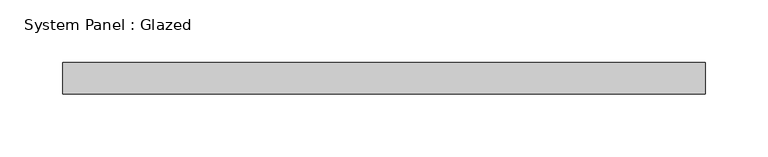
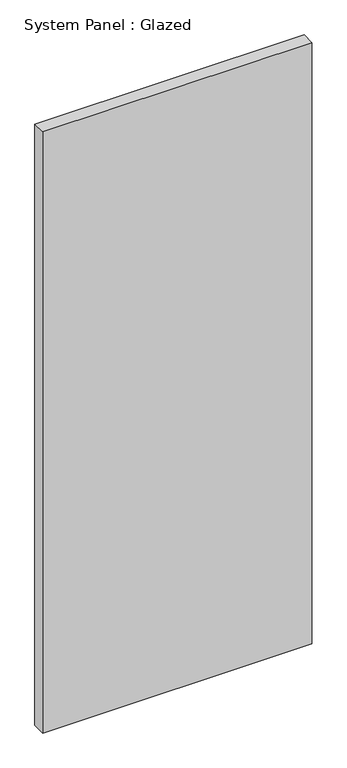
"""IFC4 building model written with IfcOpenShell, lengths in millimetres: plate geometry, System Panel : Glazed."""

from ifc_helpers import new_model, si_unit, origin, origin_with_axes, place, context, project, spatial, polyline, outline, extrude, source, transform, mapped, element, save


def system_panel_glazed_2d65dcb0(model_context):
    return source(origin(), model_context, "Body", "SweptSolid", [
        extrude(outline(polyline([(257.175, 19.05), (-257.175, 19.05), (-257.175, 44.45), (257.175, 44.45), (257.175, 19.05)])), origin_with_axes(), (0.0, 0.0, 1.0), 1214.7662723),
    ])


if __name__ == "__main__":
    model = new_model("IFC4")
    model_context = context("Model", 3, world=origin())
    ifc_project = project(units=[si_unit("LENGTHUNIT", "METRE", prefix="MILLI")], contexts=[model_context])
    site = spatial("IfcSite", under=ifc_project)
    building = spatial("IfcBuilding", under=site)
    placement = place(None, origin())
    system_panel_glazed_shape = system_panel_glazed_2d65dcb0(model_context)
    element("IfcPlate", 1, ObjectType="System Panel : Glazed", at=placement, inside=building, context=model_context, shape_type="MappedRepresentation", body=[
        mapped(system_panel_glazed_shape, transform((0.0, 0.0, 0.0), x_axis=(1.0, 0.0, 0.0), y_axis=(0.0, 1.0, 0.0), z_axis=(0.0, 0.0, 1.0))),
    ])
    save(model, "model.ifc")

# Revit data of these elements
# Type "System Panel : Glazed"
#   Construction Type Id = "GSP4R"
#   Analytic Construction = "1/8 in Pilkington single glazing"
#   Visual Light Transmittance = 0.9
#   Solar Heat Gain Coefficient = 0.86
#   Heat Transfer Coefficient (U) = 1.18115 BTU/(h·ft²·°F)
#   Define Thermal Properties by = 1
# Element 1 (IfcPlate, "System Panel : Glazed")
#   Materials on its faces: "Glass"
# Materials
#   "Glass": class "Glass", colour RGB 0 128 192, transparency 0.75, Description = "Soda Lime Glass", Cost = 0
